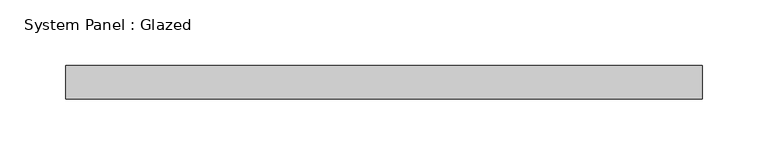
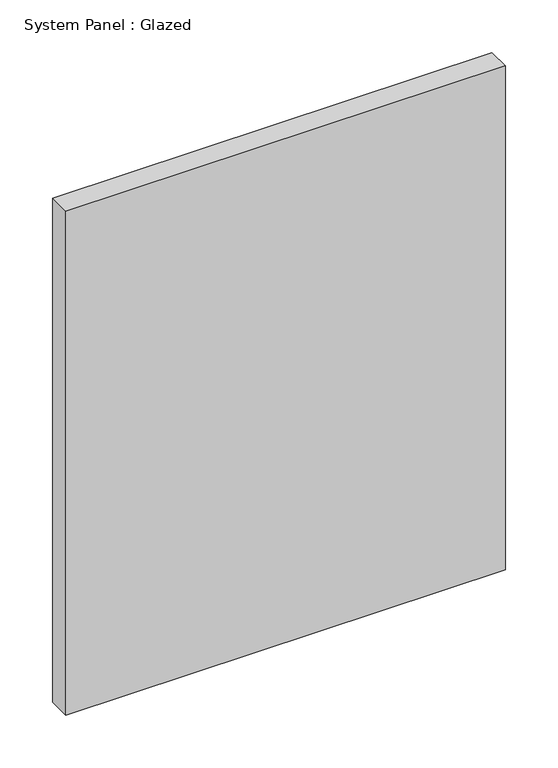
"""IFC4 building model written with IfcOpenShell, lengths in millimetres: plate geometry, System Panel : Glazed."""

from ifc_helpers import new_model, si_unit, origin, origin_with_axes, place, context, project, spatial, polyline, outline, extrude, source, transform, mapped, element, save


def system_panel_glazed_e612b4c2(model_context):
    return source(origin(), model_context, "Body", "SweptSolid", [
        extrude(outline(polyline([(241.3, 19.05), (-241.3, 19.05), (-241.3, 44.45), (241.3, 44.45), (241.3, 19.05)])), origin_with_axes(), (0.0, 0.0, 1.0), 584.9136426),
    ])


if __name__ == "__main__":
    model = new_model("IFC4")
    model_context = context("Model", 3, world=origin())
    ifc_project = project(units=[si_unit("LENGTHUNIT", "METRE", prefix="MILLI")], contexts=[model_context])
    site = spatial("IfcSite", under=ifc_project)
    building = spatial("IfcBuilding", under=site)
    placement = place(None, origin())
    system_panel_glazed_shape = system_panel_glazed_e612b4c2(model_context)
    element("IfcPlate", 1, ObjectType="System Panel : Glazed", at=placement, inside=building, context=model_context, shape_type="MappedRepresentation", body=[
        mapped(system_panel_glazed_shape, transform((0.0, 0.0, 0.0), x_axis=(1.0, 0.0, 0.0), y_axis=(0.0, 1.0, 0.0), z_axis=(0.0, 0.0, 1.0))),
    ])
    save(model, "model.ifc")

# Revit data of these elements
# Type "System Panel : Glazed"
#   Construction Type Id = "GSP4R"
#   Analytic Construction = "1/8 in Pilkington single glazing"
#   Visual Light Transmittance = 0.9
#   Solar Heat Gain Coefficient = 0.86
#   Heat Transfer Coefficient (U) = 1.18115 BTU/(h·ft²·°F)
#   Define Thermal Properties by = 1
# Element 1 (IfcPlate, "System Panel : Glazed")
#   Materials on its faces: "Glass"
# Materials
#   "Glass": class "Glass", colour RGB 0 128 192, transparency 0.75, Description = "Soda Lime Glass", Cost = 0
